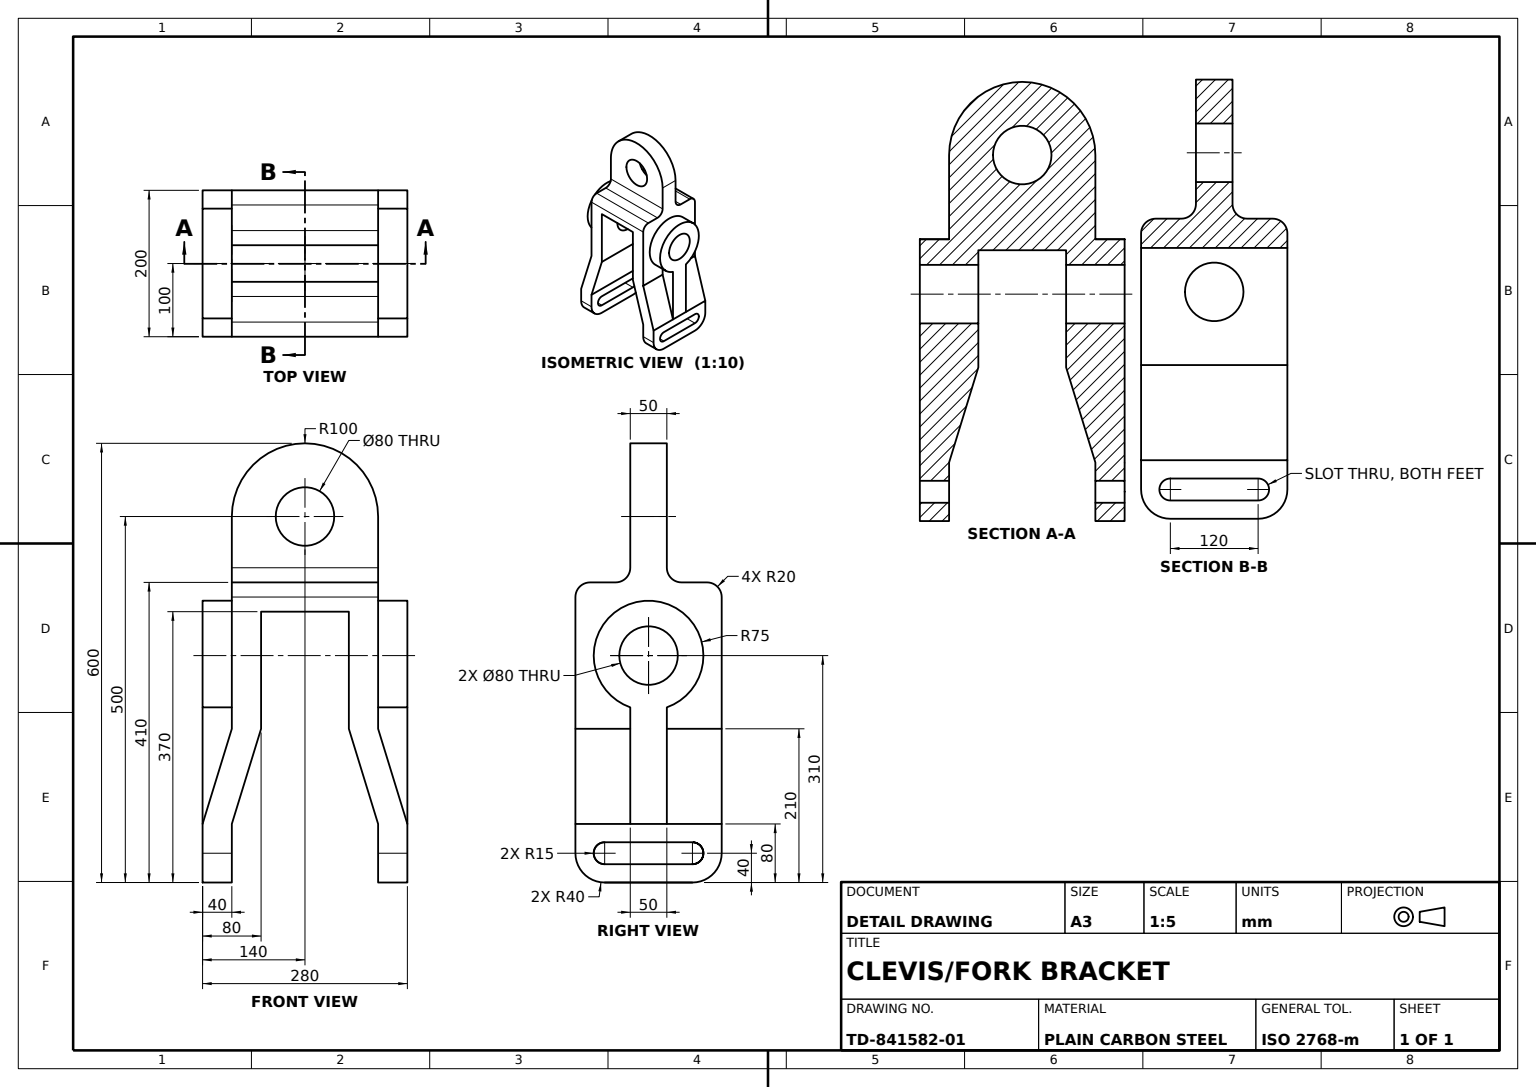
SolidWorks part; units mm, degrees
material "Plain Carbon Steel"
ref_plane "Front Plane" through (0, 0, 0) normal (0, 0, 1) x (1, 0, 0)
ref_plane "Top Plane" through (0, 0, 0) normal (0, 1, 0) x (1, 0, 0)
ref_plane "Right Plane" through (0, 0, 0) normal (1, 0, 0) x (0, 0, -1)
sketch "Fork Profile Sketch" plane through (0, 0, 0) normal (0, 0, 1) x (1, 0, 0)
  line L0 (0, 0) -> (-100, 0)
  line L1 (-100, 0) -> (-100, -200)
  line L2 (-139.9932, -330) -> (-100, -200)
  line L3 (-139.9932, -330) -> (-139.9932, -410)
  line L4 (0, 0) -> (100, 0)
  line L5 (100, 0) -> (100, -200)
  line L6 (100, -200) -> (139.9932, -330)
  line L7 (139.9932, -330) -> (139.9932, -410)
  line L8 (-139.9932, -410) -> (-99.9932, -410)
  line L9 (-99.9932, -410) -> (-99.9932, -330)
  line L10 (-99.9932, -330) -> (-60, -200)
  line L11 (-60, -200) -> (-60, -40)
  line L12 (139.9932, -410) -> (99.9932, -410)
  line L13 (99.9932, -410) -> (99.9932, -330)
  line L14 (99.9932, -330) -> (60, -200)
  line L15 (60, -200) -> (60, -40)
  line L16 (60, -40) -> (-60, -40)
  point P7 (-100, -200)
  point P12 (100, -200)
  dimension "D1" = 17.1
  dimension "D2" = 100
  dimension "D3" = 200
  dimension "D4" = 330
  dimension "D5" = 80
  dimension "D6" = 17.1
  dimension "D7" = 100
  dimension "D8" = 200
  dimension "D9" = 330
  dimension "D10" = 40
  dimension "D11" = 40
  dimension "D12" = 80
  dimension "D13" = 160
  dimension "D14" = 80
  dimension "D15" = 40
  dimension "D16" = 80
  dimension "D17" = 160
extrude "Fork Body" add sketch "Fork Profile Sketch" against normal blind 200
ref_plane "Side Boss Plane A" through (140, 0, 0) normal (1, 0, 0) x (0, 0, -1)
sketch "Side Boss A Sketch" plane through (140, 0, 0) normal (1, 0, 0) x (0, 0, -1)
  line L0 (200, -330) -> (0, -330) construction
  line L2 (75, -170.7107) -> (75, -330)
  line L3 (75, -330) -> (125, -330)
  line L4 (125, -170.7107) -> (125, -330)
  arc A0 (125, -170.7107) -> (75, -170.7107) centre (100, -100) ccw
  circle A1 centre (100, -100) radius 40
  dimension "D1" = 150
  dimension "D2" = 80
  dimension "D3" = 100
  dimension "D4" = 100
  dimension "D5" = 75
  dimension "D6" = 75
extrude "Side Boss A" add sketch "Side Boss A Sketch" against normal blind 40
ref_plane "Side Boss Plane B" through (-140, 0, 0) normal (1, 0, 0) x (0, 0, -1)
sketch "Side Boss B Sketch" plane through (-140, 0, 0) normal (1, 0, 0) x (0, 0, -1)
  line L0 (200, -330) -> (0, -330) construction
  line L2 (125, -170.7107) -> (125, -330)
  line L3 (125, -330) -> (75, -330)
  line L4 (75, -170.7107) -> (75, -330)
  arc A0 (125, -170.7107) -> (75, -170.7107) centre (100, -100) ccw
  circle A1 centre (100, -100) radius 40
  dimension "D1" = 150
  dimension "D2" = 80
  dimension "D3" = 100
  dimension "D4" = 100
  dimension "D5" = 75
  dimension "D6" = 75
extrude "Side Boss B" add sketch "Side Boss B Sketch" along normal blind 40
sketch "Pivot Bore Sketch" plane through (100, 0, 0) normal (1, 0, 0) x (0, 0, -1)
  circle A0 centre (100, -100) radius 40
  dimension "D1" = 80
extrude "Pivot Bore Ø80" cut sketch "Pivot Bore Sketch" against normal through all
ref_plane "Top Lug Plane" through (0, 0, -100) normal (0, 0, 1) x (1, 0, 0)
sketch "Top Lug Sketch" plane through (0, 0, -100) normal (0, 0, 1) x (1, 0, 0)
  line L0 (-100, 90) -> (-100, 0)
  line L1 (-100, 0) -> (100, 0)
  line L2 (100, 0) -> (100, 90)
  arc A0 (100, 90) -> (-100, 90) centre (0, 90) ccw
  circle A1 centre (0, 90) radius 40
  dimension "D1" = 200
  dimension "D4" = 80
  dimension "D2" = 90
  dimension "D3" = 0
  dimension "D5" = 90
  dimension "D6" = 200
extrude "Top Lug" add sketch "Top Lug Sketch" along normal mid plane 50
fillet "Top Lug Blend R20" radius 20 4 edges at (0, 0, -125) (0, 0, -200) (0, 0, 0) (0, 0, -75)
fillet "Fork Fillet R40 A" radius 40 1 edges at (119.9932, -410, 0)
fillet "Fork Fillet R40 B" radius 40 1 edges at (119.9932, -410, -200)
fillet "Fork Fillet R40 C" radius 40 1 edges at (-119.9932, -410, 0)
fillet "Fork Fillet R40 D" radius 40 1 edges at (-119.9932, -410, -200)
sketch "Foot Slot Sketch" plane through (139.9932, 0, 0) normal (1, 0, 0) x (0, 0, -1)
  line L0 (40, -370) -> (160, -370) construction
  line L1 (40, -355) -> (160, -355)
  line L2 (40, -385) -> (160, -385)
  arc A0 (40, -355) -> (40, -385) centre (40, -370) ccw
  arc A1 (160, -385) -> (160, -355) centre (160, -370) ccw
  point P3 (100, -370)
  dimension "D1" = 15
  dimension "D2" = 120
extrude "Foot Slots 15x120" cut sketch "Foot Slot Sketch" against normal through all
